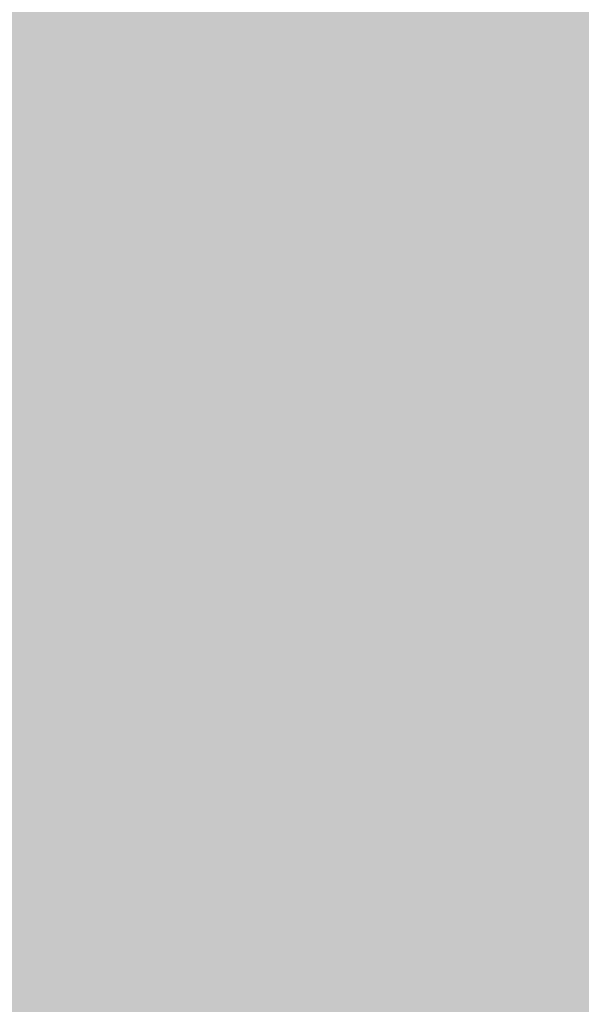
# Model space of a CAD drawing. Units: inches. Extents: x 2083 to 3317, y 1141 to 2115.
# Tile 177 of 256: x 3126.89136 to 3126.92826, y 1263.29018 to 1263.35483. Entities that reach past the tile are written whole.
import ezdxf

# ---------------------------------------------------------------- set-up
doc = ezdxf.new("R2010")
doc.units = ezdxf.units.IN
doc.layers.add('A-ANNO-DIMS', color=2, linetype='Continuous', lineweight=18)
doc.layers.add('A-WALL-PATT', color=251, linetype='Continuous', lineweight=13, true_color=0x636466)
doc.styles.get("Standard").update_dxf_attribs({"font": 'arial.ttf'})
doc.dimstyles.new('ISO-25', dxfattribs={"dimtxt": 12, "dimasz": 12, "dimexe": 1.25, "dimexo": 0.625, "dimtad": 1, "dimlunit": 3, "dimtxsty": 'Standard', "dimcen": 2.5, "dimadec": 0, "dimazin": 0, "dimtfac": 1, "dimtmove": 0, "dimatfit": 3, "dimfxl": 1, "dimarcsym": 0})

# ---------------------------------------------------------------- blocks, each defined once
blk = doc.blocks.new('*D26')
at = {"layer": 'A-ANNO-DIMS', "color": 0, "lineweight": -2, "transparency": 16777216}
for p, q in [((3088.985844, 1274.915092), (3088.985844, 1270.951963)), ((3111.240037, 1274.915092), (3111.240037, 1270.951963)), ((3076.985844, 1272.201963), (2840.262447, 1272.201963)), ((3111.240037, 1272.201963), (3088.985844, 1272.201963)), ((3123.240037, 1272.201963), (3135.240037, 1272.201963))]:
    blk.add_line(p, q, dxfattribs=at)
at = {"layer": 'A-ANNO-DIMS', "color": 0, "transparency": 16777216}
for points in [[(3076.985844, 1274.201963), (3076.985844, 1270.201963), (3088.985844, 1272.201963)], [(3123.240037, 1274.201963), (3123.240037, 1270.201963), (3111.240037, 1272.201963)]]:
    blk.add_solid(points, dxfattribs=at)
at = {"layer": 'Defpoints', "color": 0, "transparency": 16777216}
for p in [(3088.985844, 1275.540092), (3111.240037, 1275.540092), (3088.985844, 1272.201963)]:
    blk.add_point(p, dxfattribs=at)
at = {"layer": 'A-ANNO-DIMS', "color": 0, "transparency": 16777216, "insert": (2952.624146, 1279.031602), "char_height": 12, "attachment_point": 5}
blk.add_mtext('NIGHTSTAND 1\'-10 1/2" TYP.', dxfattribs=at)
blk = doc.blocks.new('*D27')
at = {"layer": 'A-ANNO-DIMS', "color": 0, "lineweight": -2, "transparency": 16777216}
for p, q in [((3114.578165, 1309.794285), (3114.578165, 1321.794285)), ((3111.865037, 1297.794285), (3115.828165, 1297.794285)), ((3114.578165, 1297.794285), (3114.578165, 1275.540092)), ((3111.865037, 1275.540092), (3115.828165, 1275.540092)), ((3114.578165, 1263.540092), (3114.578165, 1140.988591))]:
    blk.add_line(p, q, dxfattribs=at)
at = {"layer": 'A-ANNO-DIMS', "color": 0, "transparency": 16777216}
for points in [[(3112.578165, 1309.794285), (3116.578165, 1309.794285), (3114.578165, 1297.794285)], [(3112.578165, 1263.540092), (3116.578165, 1263.540092), (3114.578165, 1275.540092)]]:
    blk.add_solid(points, dxfattribs=at)
at = {"layer": 'Defpoints', "color": 0, "transparency": 16777216}
for p in [(3111.240037, 1297.794285), (3111.240037, 1275.540092), (3114.578165, 1275.540092)]:
    blk.add_point(p, dxfattribs=at)
at = {"layer": 'A-ANNO-DIMS', "color": 0, "transparency": 16777216, "insert": (3107.748527, 1196.264342), "char_height": 12, "attachment_point": 5, "rotation": 90}
blk.add_mtext('1\'-10 1/2" TYP.', dxfattribs=at)

msp = doc.modelspace()

# ---------------------------------------------------------------- hatches: boundary and pattern name
at = {"layer": 'A-WALL-PATT'}
h = msp.add_hatch(color=256, dxfattribs=at)
h.dxf.hatch_style = 1
h.paths.add_polyline_path([(3126.959783, 2020.76136), (2748.959783, 2020.76136), (2604.959783, 2020.76136), (2226.959783, 2020.76136), (2226.959783, 1702.76136), (2466.959783, 1702.76136), (2466.959783, 1582.76136), (2418.959783, 1582.76136), (2418.959783, 1477.76136), (2226.959783, 1477.76136), (2226.959783, 1263.26136), (2544.959783, 1263.26136), (2544.959783, 1411.76136), (2604.959783, 1411.76136), (2685.959783, 1411.76136), (2685.959783, 1420.76136), (2604.959783, 1420.76136), (2604.959783, 1573.76136), (2604.959783, 1702.76136), (2604.959783, 2011.76136), (2748.959783, 2011.76136), (2748.959783, 1702.76136), (2862.959783, 1702.76136), (2862.959783, 1621.76136), (2871.959783, 1621.76136), (2871.959783, 1702.76136), (2883.959783, 1702.76136), (2883.959783, 1706.939459, -0.026459), (2883.959783, 1711.76136), (2757.959783, 1711.76136), (2757.959783, 1807.76136), (2787.959783, 1807.76136), (2787.959783, 1812.26136), (2757.959783, 1812.26136), (2757.959783, 2011.76136), (2877.959783, 2011.76136), (2877.959783, 1812.26136), (2847.959783, 1812.26136), (2847.959783, 1807.76136), (2889.835742, 1807.76136), (2889.835742, 1812.26136), (2882.459783, 1812.26136), (2882.459783, 2011.76136), (3117.959783, 2011.76136), (3117.959783, 1812.26136), (2937.835742, 1812.26136), (2937.835742, 1807.76136), (2995.709783, 1807.76136), (2995.709783, 1796.117666), (3000.209783, 1796.117666), (3000.209783, 1807.76136), (3117.959783, 1807.76136), (3117.959783, 1711.76136), (3000.209783, 1711.76136), (3000.209783, 1760.117666), (2998.572705, 1760.117666, -0.020711), (2995.709783, 1760.117666), (2995.709783, 1711.76136), (2931.959783, 1711.76136), (2931.959783, 1702.76136), (3126.959783, 1702.76136)])
h.paths.add_polyline_path([(2471.459783, 2011.76136), (2471.459783, 1810.01136), (2462.716936, 1810.01136), (2462.716936, 1805.51136), (2505.959783, 1805.51136), (2505.959783, 1810.01136), (2475.959783, 1810.01136), (2475.959783, 2011.76136), (2595.959783, 2011.76136), (2595.959783, 1810.01136), (2565.959783, 1810.01136), (2565.959783, 1805.51136), (2595.959783, 1805.51136), (2595.959783, 1711.76136), (2235.959783, 1711.76136), (2235.959783, 1805.51136), (2353.709783, 1805.51136), (2353.709783, 1796.054162), (2358.209783, 1796.054162), (2358.209783, 1805.51136), (2414.716936, 1805.51136), (2414.716936, 1810.01136), (2235.959783, 1810.01136), (2235.959783, 2011.76136)], flags=16)
h.paths.add_polyline_path([(2270.204734, 1994.610008), (2270.204734, 1970.610008), (2246.204734, 1970.610008), (2246.204734, 1994.610008)], flags=0)
edge = h.paths.add_edge_path(flags=0)
edge.add_ellipse((2332.027391, 1899.798176), major_axis=(-3.042994, 3.042994), ratio=0.16825245, start_angle=-161.332166, end_angle=-156.307114, ccw=False)
edge.add_ellipse((2333.082037, 1898.74353), major_axis=(-1.054646, 1.054646), ratio=0.4535321, start_angle=-123.371019, end_angle=-94.159107)
edge = h.paths.add_edge_path(flags=0)
edge.add_ellipse((2332.027391, 1968.87629), major_axis=(3.042994, 3.042994), ratio=0.16825245, start_angle=18.667834, end_angle=23.692886)
edge.add_spline(control_points=[(2332.925596, 1970.691105), (2332.226768, 1970.3361), (2330.893709, 1969.658905), (2328.41308, 1970.932138), (2327.203934, 1967.748712), (2324.709596, 1969.955589), (2322.532822, 1967.012354), (2320.012846, 1971.295812), (2317.680308, 1968.157845), (2316.040526, 1967.102047), (2315.426904, 1966.809602)], knot_values=[0, 0, 0, 0, 2.267059, 4.324559, 6.685584, 8.878641, 11.121502, 14.300359, 17.755284, 19.732645, 19.732645, 19.732645, 19.732645], degree=3, periodic=0)
edge.add_ellipse((2332.027391, 1968.87629), major_axis=(3.042994, 3.042994), ratio=0.16825245, start_angle=18.667834, end_angle=23.692886, ccw=False)
edge.add_ellipse((2333.082037, 1969.930936), major_axis=(1.054646, 1.054646), ratio=0.4535321, start_angle=56.628981, end_angle=85.840893, ccw=False)
edge = h.paths.add_edge_path(flags=0)
edge.add_spline(control_points=[(2296.428287, 1967.987908), (2293.627804, 1965.336314), (2287.703624, 1959.727094), (2299.74386, 1949.995699), (2294.532591, 1935.668528), (2290.573228, 1920.603512), (2293.394124, 1909.973691), (2296.185407, 1904.966543)], knot_values=[0.099185, 0.099185, 0.099185, 0.099185, 0.345301, 0.619822, 0.982653, 1.386093, 1.810555, 1.810555, 1.810555, 1.810555], degree=3, periodic=0)
edge.add_spline(control_points=[(2296.185407, 1904.966543), (2297.383582, 1902.6193), (2298.000969, 1901.949312), (2298.55297, 1901.468155)], knot_values=[0.006246, 0.006246, 0.006246, 0.006246, 0.055476, 0.055476, 0.055476, 0.055476], degree=3, periodic=0)
edge.add_spline(control_points=[(2298.55297, 1901.468155), (2297.258612, 1900.923224), (2295.225294, 1900.232126), (2293.060229, 1900.614205), (2292.101423, 1900.788415), (2292.089578, 1900.790568)], knot_values=[0.312835, 0.312835, 0.312835, 0.312835, 0.40178, 0.474987, 0.475903, 0.475903, 0.475903, 0.475903], degree=3, periodic=0)
edge.add_arc((2292.793646, 1904.664109), 3.937008, 215.420897, 259.698179, ccw=False)
edge.add_spline(control_points=[(2289.585314, 1902.382304), (2289.476652, 1902.535087), (2289.36848, 1902.688035), (2289.260865, 1902.84117)], knot_values=[0.102872, 0.102872, 0.102872, 0.102872, 0.116896, 0.116896, 0.116896, 0.116896], degree=3, periodic=0)
edge.add_spline(control_points=[(2289.260865, 1902.84117), (2288.686604, 1902.550192), (2287.640048, 1902.019902), (2285.881337, 1901.873954), (2283.852972, 1901.504352), (2281.719987, 1899.710538), (2278.466991, 1899.492942), (2276.157136, 1901.883202), (2272.258953, 1899.804071), (2267.777605, 1901.843183), (2262.243882, 1900.184033), (2257.414927, 1901.782061), (2254.318374, 1900.72612), (2253.178285, 1900.337343)], knot_values=[0, 0, 0, 0, 1.907977, 3.477176, 5.261074, 7.972851, 11.680248, 13.717921, 16.939592, 22.789562, 27.502503, 33.595215, 37.145618, 37.145618, 37.145618, 37.145618], degree=3, periodic=0)
edge.add_line((2253.178285, 1900.337343), (2250.24424, 1902.84117))
edge.add_line((2250.24424, 1902.84117), (2250.24424, 1965.833296))
edge.add_line((2250.24424, 1965.833296), (2253.178285, 1968.337123))
edge.add_spline(control_points=[(2253.178285, 1968.337123), (2254.318374, 1967.948346), (2257.414927, 1966.892405), (2262.243882, 1968.490433), (2267.777605, 1966.831283), (2271.52673, 1968.537217), (2273.875914, 1967.828289), (2274.206701, 1967.727642)], knot_values=[0, 0, 0, 0, 0.09018, 0.244935, 0.364644, 0.513233, 0.537855, 0.537855, 0.537855, 0.537855], degree=3, periodic=0)
edge.add_arc((2274.352887, 1963.793349), 3.937008, 72.051134, 92.127949, ccw=False)
edge.add_arc((2281.296933, 1985.230003), 18.596298, 252.0511336, 288.5657217)
edge.add_arc((2292.316717, 1956.02888), 12.646081, 71.0267879, 113.7782184, ccw=False)
edge = h.paths.add_edge_path(flags=0)
edge.add_spline(control_points=[(2274.899415, 1951.856195), (2275.066156, 1951.616592), (2275.232687, 1951.376588), (2275.397987, 1951.135855)], knot_values=[1.409916, 1.409916, 1.409916, 1.409916, 1.43159, 1.43159, 1.43159, 1.43159], degree=3, periodic=0)
edge.add_spline(control_points=[(2275.397987, 1951.135855), (2275.792106, 1950.561885), (2276.179231, 1949.983774), (2276.545546, 1949.397103)], knot_values=[1.358238, 1.358238, 1.358238, 1.358238, 1.409916, 1.409916, 1.409916, 1.409916], degree=3, periodic=0)
edge.add_line((2276.545546, 1949.397103), (2277.437289, 1947.862185))
edge.add_spline(control_points=[(2277.437289, 1947.862185), (2276.303834, 1945.673115), (2274.639698, 1942.426882), (2274.631615, 1938.0939), (2272.799124, 1930.85155), (2274.356426, 1943.897046), (2275.947681, 1947.923356), (2276.545546, 1949.397103)], knot_values=[0.005632, 0.005632, 0.005632, 0.005632, 0.186014, 0.266002, 0.357087, 0.59639, 0.739732, 0.739732, 0.739732, 0.739732], degree=3, periodic=0)
edge.add_spline(control_points=[(2276.545546, 1949.397103), (2276.179231, 1949.983774), (2275.792106, 1950.561885), (2275.397987, 1951.135855)], knot_values=[1.358238, 1.358238, 1.358238, 1.358238, 1.409916, 1.409916, 1.409916, 1.409916], degree=3, periodic=0)
edge.add_spline(control_points=[(2275.397987, 1951.135855), (2274.9425, 1950.080452), (2274.20776, 1948.025272), (2273.934602, 1944.851477), (2272.468534, 1937.627489), (2273.466216, 1945.696466), (2274.700615, 1951.059472), (2274.899415, 1951.856195)], knot_values=[0.104364, 0.104364, 0.104364, 0.104364, 0.189636, 0.269624, 0.36071, 0.600013, 0.644622, 0.644622, 0.644622, 0.644622], degree=3, periodic=0)
h.paths.add_polyline_path([(2269.167514, 1963.127573, -0.357527), (2268.170633, 1960.97637, -0.092561), (2268.170633, 1939.436325, -0.357527), (2269.167514, 1937.285122, -0.357527), (2267.01631, 1938.282002, -0.164785), (2254.685581, 1938.282002, -0.357527), (2252.534378, 1937.285122, -0.357527), (2253.531259, 1939.436325, -0.092561), (2253.531259, 1960.97637, -0.357527), (2252.534378, 1963.127573, -0.357527), (2254.685581, 1962.130692, -0.164785), (2267.01631, 1962.130692, -0.357527)], flags=0)
h.paths.add_polyline_path([(2248.874068, 1967.8018), (2248.874068, 1957.02771), (2249.457783, 1957.02771), (2249.457783, 1911.646756), (2248.874068, 1911.646756), (2248.874068, 1900.872666), (2246.511863, 1900.872666, 0.197327), (2244.149658, 1902.456873), (2244.149658, 1966.217592, 0.197327), (2246.511863, 1967.8018)], flags=0)
h.paths.add_polyline_path([(2269.167514, 1931.389344, -0.357527), (2268.170633, 1929.238141, -0.092561), (2268.170633, 1907.698096, -0.357527), (2269.167514, 1905.546893, -0.357527), (2267.01631, 1906.543774, -0.164785), (2254.685581, 1906.543774, -0.357527), (2252.534378, 1905.546893, -0.357527), (2253.531259, 1907.698096, -0.092561), (2253.531259, 1929.238141, -0.357527), (2252.534378, 1931.389344, -0.357527), (2254.685581, 1930.392463, -0.164785), (2267.01631, 1930.392463, -0.357527)], flags=0)
edge = h.paths.add_edge_path(flags=0)
edge.add_spline(control_points=[(2276.196858, 1906.723702), (2276.168144, 1909.028928), (2276.114049, 1913.371852), (2270.598417, 1924.924978), (2273.905175, 1919.012779), (2275.921711, 1916.262063), (2275.47457, 1912.402149), (2277.257874, 1910.380621), (2276.696044, 1908.225036), (2276.646218, 1906.813023), (2276.617825, 1906.008407)], knot_values=[0, 0, 0, 0, 8.61026, 16.221274, 18.843057, 23.804898, 27.440828, 29.356102, 31.203478, 33.650687, 33.650687, 33.650687, 33.650687], degree=3, periodic=0)
edge.add_spline(control_points=[(2276.617825, 1906.008407), (2276.623313, 1905.624144), (2276.497738, 1904.628661), (2275.441779, 1903.854725), (2274.937314, 1903.08045), (2274.85908, 1902.84117)], knot_values=[0.156488, 0.156488, 0.156488, 0.156488, 0.184398, 0.231376, 0.250598, 0.250598, 0.250598, 0.250598], degree=3, periodic=0)
edge.add_line((2274.85908, 1902.84117), (2276.50598, 1902.84117))
edge.add_spline(control_points=[(2276.50598, 1902.84117), (2276.788308, 1903.08494), (2277.665071, 1904.125196), (2278.249538, 1904.340738), (2277.653872, 1908.527387), (2278.15567, 1906.227808), (2278.100464, 1905.285948), (2278.846675, 1904.069005), (2277.856785, 1903.414948), (2277.874191, 1902.99105), (2277.903562, 1902.84117)], knot_values=[0.059574, 0.059574, 0.059574, 0.059574, 0.080753, 0.103741, 0.16972, 0.176036, 0.207137, 0.240474, 0.262341, 0.27366, 0.27366, 0.27366, 0.27366], degree=3, periodic=0)
edge.add_line((2277.903562, 1902.84117), (2280.029825, 1902.84117))
edge.add_spline(control_points=[(2280.029825, 1902.84117), (2279.888221, 1903.088398), (2279.499257, 1903.981551), (2280.152284, 1905.939349), (2278.103615, 1909.657757), (2279.762395, 1907.185285), (2280.3279, 1904.874861), (2280.485109, 1903.48959), (2281.463269, 1903.249432), (2281.758343, 1902.936497), (2281.834036, 1902.84117)], knot_values=[0.013856, 0.013856, 0.013856, 0.013856, 0.034874, 0.088867, 0.107879, 0.126738, 0.158714, 0.193757, 0.217487, 0.226722, 0.226722, 0.226722, 0.226722], degree=3, periodic=0)
edge.add_spline(control_points=[(2281.834036, 1902.84117), (2281.787535, 1902.826703), (2281.647022, 1902.782988), (2281.395527, 1902.85949), (2281.088077, 1902.985242), (2280.720683, 1903.060902), (2280.333451, 1903.025726), (2280.124767, 1902.898879), (2280.029825, 1902.84117)], knot_values=[0, 0, 0, 0, 0.14413, 0.435517, 0.749276, 1.153046, 1.548371, 1.878348, 1.878348, 1.878348, 1.878348], degree=3, periodic=0)
edge.add_line((2280.029825, 1902.84117), (2277.903562, 1902.84117))
edge.add_spline(control_points=[(2277.903562, 1902.84117), (2277.892855, 1902.795855), (2277.865396, 1902.679637), (2277.607479, 1902.687483), (2277.27405, 1902.8007), (2276.837921, 1902.619775), (2276.583807, 1902.789261), (2276.50598, 1902.84117)], knot_values=[0, 0, 0, 0, 0.127189, 0.326199, 0.628009, 1.24357, 1.515331, 1.515331, 1.515331, 1.515331], degree=3, periodic=0)
edge.add_line((2276.50598, 1902.84117), (2274.85908, 1902.84117))
edge.add_spline(control_points=[(2274.85908, 1902.84117), (2274.814437, 1902.898587), (2274.72513, 1903.013446), (2274.493477, 1903.118968), (2274.244285, 1902.960539), (2273.937121, 1903.184942), (2273.614039, 1902.983143), (2273.408316, 1902.883045), (2273.322254, 1902.84117)], knot_values=[0, 0, 0, 0, 0.21843, 0.436957, 0.687977, 0.990379, 1.398396, 1.69185, 1.69185, 1.69185, 1.69185], degree=3, periodic=0)
edge.add_spline(control_points=[(2273.322254, 1902.84117), (2273.61674, 1903.445692), (2274.273998, 1904.538253), (2276.027239, 1904.573702), (2276.206963, 1906.583637), (2276.196858, 1906.723702)], knot_values=[0.012227, 0.012227, 0.012227, 0.012227, 0.059472, 0.106218, 0.134458, 0.134458, 0.134458, 0.134458], degree=3, periodic=0)
h.paths.add_polyline_path([(2270.776054, 1897.789828), (2270.776054, 1873.789828), (2246.776054, 1873.789828), (2246.776054, 1897.789828)], flags=0)
h.paths.add_polyline_path([(2353.709783, 1760.005059), (2353.709783, 1760.054162), (2358.209783, 1760.054162, -0.033729)], flags=0)
h.paths.add_polyline_path([(2321.819119, 1737.529186), (2341.995327, 1737.529186, -0.414214), (2343.203273, 1736.321241), (2343.203273, 1721.020596, -0.414214), (2341.995327, 1719.812651), (2321.819119, 1719.812651, -0.414214), (2320.611173, 1721.020596), (2320.611173, 1736.321241, -0.414214)], flags=0)
h.paths.add_polyline_path([(2324.23501, 1736.321241), (2339.579436, 1736.321241, -0.414214), (2341.995327, 1733.905349), (2341.995327, 1725.44973, -0.414214), (2339.579436, 1723.033839), (2333.680588, 1723.033839), (2333.845317, 1722.045467, -0.870646), (2335.425399, 1721.825893, -0.767327), (2333.922694, 1721.423245), (2331.291024, 1721.423245, -0.767327), (2329.788319, 1721.825893, -0.870646), (2331.368401, 1722.045467), (2331.53313, 1723.033839), (2324.23501, 1723.033839, -0.414214), (2321.819119, 1725.44973), (2321.819119, 1733.905349, -0.414214)], flags=0)
h.paths.add_polyline_path([(2570.483789, 1928.615444), (2589.683789, 1928.615444), (2590.168829, 1928.615444), (2590.168829, 1904.993397), (2570.483789, 1904.993397)], flags=0)
h.paths.add_polyline_path([(2574.447324, 1927.263822, -1), (2572.828836, 1927.263822, -1)], flags=0)
h.paths.add_polyline_path([(2573.089867, 1926.940877), (2573.925032, 1927.776042), (2574.147743, 1927.553332), (2573.312577, 1926.718166)], flags=0)
h.paths.add_polyline_path([(2578.779065, 1919.729618, -1), (2571.591663, 1919.729618, -1)], flags=0)
h.paths.add_polyline_path([(2578.385364, 1919.729618, -1), (2571.985364, 1919.729618, -1)], flags=0)
h.paths.add_polyline_path([(2331.595764, 1729.476216, -1), (2333.617954, 1729.476216, -1)], flags=0)
h.paths.add_polyline_path([(2578.034228, 1927.263822, -1), (2576.41574, 1927.263822, -1)], flags=0)
h.paths.add_polyline_path([(2576.688851, 1927.531089), (2576.911562, 1927.753799), (2577.746728, 1926.918634), (2577.524017, 1926.695923)], flags=0)
h.paths.add_polyline_path([(2578.139065, 1909.859539, -1), (2572.231663, 1909.859539, -1)], flags=0)
h.paths.add_polyline_path([(2577.745364, 1909.859539, -1), (2572.625364, 1909.859539, -1)], flags=0)
h.paths.add_polyline_path([(2583.797718, 1927.263822, -1), (2582.179229, 1927.263822, -1)], flags=0)
h.paths.add_polyline_path([(2582.718649, 1927.753799), (2583.553814, 1926.918634), (2583.331103, 1926.695923), (2582.495938, 1927.531089)], flags=0)
h.paths.add_polyline_path([(2582.495938, 1927.531089), (2582.718649, 1927.753799), (2583.553814, 1926.918634), (2583.331103, 1926.695923)], flags=0)
h.paths.add_polyline_path([(2587.739065, 1920.529618, -1), (2581.831663, 1920.529618, -1)], flags=0)
h.paths.add_polyline_path([(2587.345364, 1920.529618, -1), (2582.225364, 1920.529618, -1)], flags=0)
h.paths.add_polyline_path([(2587.384622, 1927.263822, -1), (2585.766133, 1927.263822, -1)], flags=0)
h.paths.add_polyline_path([(2586.081993, 1926.980247), (2586.917158, 1927.815412), (2587.139869, 1927.592702), (2586.304703, 1926.757536)], flags=0)
h.paths.add_polyline_path([(2588.379065, 1910.659539, -1), (2581.191663, 1910.659539, -1)], flags=0)
h.paths.add_polyline_path([(2587.985364, 1910.659539, -1), (2581.585364, 1910.659539, -1)], flags=0)
h.paths.add_polyline_path([(2417.167729, 1729.477895), (2437.343937, 1729.477895, -0.414214), (2438.551883, 1728.26995), (2438.551883, 1712.969306, -0.414214), (2437.343937, 1711.76136), (2417.167729, 1711.76136, -0.414214), (2415.959783, 1712.969306), (2415.959783, 1728.26995, -0.414214)], flags=0)
h.paths.add_polyline_path([(2419.58362, 1728.26995), (2434.928046, 1728.26995, -0.414214), (2437.343937, 1725.854059), (2437.343937, 1717.39844, -0.414214), (2434.928046, 1714.982548), (2429.029199, 1714.982548), (2429.193927, 1713.994176, -0.870646), (2430.774009, 1713.774603, -0.767327), (2429.271304, 1713.371954), (2426.639634, 1713.371954, -0.767327), (2425.136929, 1713.774603, -0.870646), (2426.717011, 1713.994176), (2426.88174, 1714.982548), (2419.58362, 1714.982548, -0.414214), (2417.167729, 1717.39844), (2417.167729, 1725.854059, -0.414214)], flags=0)
h.paths.add_polyline_path([(2419.58362, 1728.26995), (2434.928046, 1728.26995, -0.414214), (2437.343937, 1725.854059), (2437.343937, 1717.39844, -0.414214), (2434.928046, 1714.982548), (2429.029199, 1714.982548), (2428.358118, 1719.009034), (2427.552821, 1719.009034), (2426.88174, 1714.982548), (2419.58362, 1714.982548, -0.414214), (2417.167729, 1717.39844), (2417.167729, 1725.854059, -0.414214)], flags=0)
h.paths.add_polyline_path([(2426.944374, 1721.424925, -1), (2428.966564, 1721.424925, -1)], flags=0)
h.paths.add_polyline_path([(2475.959783, 1702.76136), (2595.959783, 1702.76136), (2595.959783, 1582.76136), (2475.959783, 1582.76136)], flags=16)
h.paths.add_polyline_path([(2427.959783, 1573.76136), (2595.959783, 1573.76136), (2595.959783, 1468.76136), (2595.959783, 1420.76136), (2384.459783, 1420.76136), (2384.459783, 1468.76136), (2427.959783, 1468.76136)], flags=16)
h.paths.add_polyline_path([(2379.959783, 1468.76136), (2379.959783, 1420.76136), (2235.959783, 1420.76136), (2235.959783, 1468.76136)], flags=16)
h.paths.add_polyline_path([(2317.815996, 1466.695767), (2337.992205, 1466.695767, -0.414214), (2339.20015, 1465.487821), (2339.20015, 1450.187177, -0.414214), (2337.992205, 1448.979232), (2317.815996, 1448.979232, -0.414214), (2316.608051, 1450.187177), (2316.608051, 1465.487821, -0.414214)], flags=0)
h.paths.add_polyline_path([(2320.231887, 1465.487821), (2335.576313, 1465.487821, -0.414214), (2337.992205, 1463.07193), (2337.992205, 1454.616311, -0.414214), (2335.576313, 1452.20042), (2329.677466, 1452.20042), (2329.842195, 1451.212047, -0.870646), (2331.422276, 1450.992474, -0.767327), (2329.919571, 1450.589826), (2327.287902, 1450.589826, -0.767327), (2325.785197, 1450.992474, -0.870646), (2327.365278, 1451.212047), (2327.530007, 1452.20042), (2320.231887, 1452.20042, -0.414214), (2317.815996, 1454.616311), (2317.815996, 1463.07193, -0.414214)], flags=0)
h.paths.add_polyline_path([(2320.231887, 1465.487821), (2335.576313, 1465.487821, -0.414214), (2337.992205, 1463.07193), (2337.992205, 1454.616311, -0.414214), (2335.576313, 1452.20042), (2329.677466, 1452.20042), (2329.006385, 1456.226905), (2328.201088, 1456.226905), (2327.530007, 1452.20042), (2320.231887, 1452.20042, -0.414214), (2317.815996, 1454.616311), (2317.815996, 1463.07193, -0.414214)], flags=0)
h.paths.add_polyline_path([(2327.592641, 1458.642796, -1), (2329.614832, 1458.642796, -1)], flags=0)
h.paths.add_polyline_path([(2244.411744, 1433.340453), (2241.920945, 1433.340453, -0.414214), (2240.017856, 1435.243542), (2240.017856, 1440.952808, -0.414211), (2241.920925, 1442.855897), (2244.411744, 1442.855897, -1.976472)], flags=0)
h.paths.add_polyline_path([(2245.356888, 1434.397536, -0.414214), (2245.356888, 1441.798814, -2.144098)], flags=0)
h.paths.add_polyline_path([(2535.959783, 1416.26136), (2535.959783, 1272.26136), (2235.959783, 1272.26136), (2235.959783, 1416.26136)], flags=16)
h.paths.add_polyline_path([(2260.119561, 1384.292841), (2260.119561, 1362.038649), (2237.865369, 1362.038649), (2237.865369, 1384.292841)], flags=0)
edge = h.paths.add_edge_path(flags=0)
edge.add_line((2318.251847, 1362.093298), (2318.145797, 1362.000973))
edge.add_ellipse((2317.445116, 1360.431044), major_axis=(2.82164, 2.82164), ratio=0.16825245, start_angle=18.667834, end_angle=20.948127, ccw=False)
edge.add_ellipse((2318.423045, 1361.408974), major_axis=(0.977929, 0.977929), ratio=0.4535321, start_angle=56.628981, end_angle=70.226201, ccw=False)
edge = h.paths.add_edge_path(flags=0)
edge.add_line((2319.10737, 1295.571078), (2319.015044, 1295.677128))
edge.add_ellipse((2317.445116, 1296.377809), major_axis=(-2.82164, 2.82164), ratio=0.16825245, start_angle=-161.332166, end_angle=-159.051873, ccw=False)
edge.add_ellipse((2318.423045, 1295.39988), major_axis=(-0.977929, 0.977929), ratio=0.4535321, start_angle=-123.371019, end_angle=-109.773799)
edge = h.paths.add_edge_path(flags=0)
edge.add_spline(control_points=[(2284.210349, 1301.170219), (2284.580688, 1300.444719), (2284.891189, 1299.892024), (2285.159553, 1299.461018)], knot_values=[0.039066, 0.039066, 0.039066, 0.039066, 0.055476, 0.055476, 0.055476, 0.055476], degree=3, periodic=0)
edge.add_line((2285.159553, 1299.461018), (2284.210349, 1301.170219))
edge = h.paths.add_edge_path(flags=0)
edge.add_line((2280.412458, 1297.298013), (2283.369991, 1297.036122))
edge.add_line((2283.369991, 1297.036122), (2286.40569, 1297.92631))
edge.add_spline(control_points=[(2286.40569, 1297.92631), (2285.305487, 1297.463119), (2284.344777, 1297.129151), (2283.369991, 1297.036122)], knot_values=[0.394369, 0.394369, 0.394369, 0.394369, 0.475903, 0.475903, 0.475903, 0.475903], degree=3, periodic=0)
edge.add_spline(control_points=[(2283.369991, 1297.036122), (2283.28139, 1297.027666), (2282.316289, 1296.957336), (2281.312502, 1297.134479), (2280.423441, 1297.296016), (2280.412458, 1297.298013)], knot_values=[0.312835, 0.312835, 0.312835, 0.312835, 0.320246, 0.393453, 0.394369, 0.394369, 0.394369, 0.394369], degree=3, periodic=0)
edge = h.paths.add_edge_path(flags=0)
edge.add_line((2284.435561, 1359.607285), (2280.446291, 1355.328047))
edge.add_line((2280.446291, 1355.328047), (2279.579987, 1351.017754))
edge.add_line((2279.579987, 1351.017754), (2282.412974, 1346.580433))
edge.add_spline(control_points=[(2282.412974, 1346.580433), (2283.153331, 1345.589236), (2284.252896, 1344.028897), (2284.801037, 1342.387167), (2284.935162, 1341.805544)], knot_values=[1.240098, 1.240098, 1.240098, 1.240098, 1.332892, 1.382712, 1.382712, 1.382712, 1.382712], degree=3, periodic=0)
edge.add_spline(control_points=[(2284.935162, 1341.805544), (2285.319108, 1340.1406), (2285.233029, 1338.409204), (2284.909938, 1336.654122)], knot_values=[1.097484, 1.097484, 1.097484, 1.097484, 1.240098, 1.240098, 1.240098, 1.240098], degree=3, periodic=0)
edge.add_spline(control_points=[(2284.909938, 1336.654122), (2284.586848, 1334.89904), (2284.026745, 1333.120272), (2283.462644, 1331.360585)], knot_values=[0.95487, 0.95487, 0.95487, 0.95487, 1.097484, 1.097484, 1.097484, 1.097484], degree=3, periodic=0)
edge.add_line((2283.462644, 1331.360585), (2281.890376, 1326.153357))
edge.add_line((2281.890376, 1326.153357), (2280.756259, 1321.056089))
edge.add_line((2280.756259, 1321.056089), (2280.299205, 1316.001977))
edge.add_line((2280.299205, 1316.001977), (2280.715933, 1310.950068))
edge.add_line((2280.715933, 1310.950068), (2282.028094, 1305.972137))
edge.add_line((2282.028094, 1305.972137), (2284.210349, 1301.170219))
edge.add_spline(control_points=[(2284.210349, 1301.170219), (2283.340731, 1302.730185), (2282.611904, 1304.336493), (2282.028094, 1305.972137)], knot_values=[0.099185, 0.099185, 0.099185, 0.099185, 0.241799, 0.241799, 0.241799, 0.241799], degree=3, periodic=0)
edge.add_spline(control_points=[(2282.028094, 1305.972137), (2281.444283, 1307.60778), (2281.005489, 1309.272759), (2280.715933, 1310.950068)], knot_values=[0.241799, 0.241799, 0.241799, 0.241799, 0.384413, 0.384413, 0.384413, 0.384413], degree=3, periodic=0)
edge.add_spline(control_points=[(2280.715933, 1310.950068), (2280.433241, 1312.587613), (2280.289386, 1314.276959), (2280.298894, 1315.962032), (2280.299205, 1316.001977)], knot_values=[0.384413, 0.384413, 0.384413, 0.384413, 0.523647, 0.527028, 0.527028, 0.527028, 0.527028], degree=3, periodic=0)
edge.add_spline(control_points=[(2280.299205, 1316.001977), (2280.312326, 1317.686955), (2280.477871, 1319.367926), (2280.756259, 1321.056089)], knot_values=[0.527028, 0.527028, 0.527028, 0.527028, 0.669642, 0.669642, 0.669642, 0.669642], degree=3, periodic=0)
edge.add_spline(control_points=[(2280.756259, 1321.056089), (2281.034648, 1322.744252), (2281.42588, 1324.439608), (2281.890376, 1326.153357)], knot_values=[0.669642, 0.669642, 0.669642, 0.669642, 0.812256, 0.812256, 0.812256, 0.812256], degree=3, periodic=0)
edge.add_spline(control_points=[(2281.890376, 1326.153357), (2282.264383, 1327.533251), (2282.78787, 1329.26181), (2283.352751, 1331.01778), (2283.462644, 1331.360585)], knot_values=[0.812256, 0.812256, 0.812256, 0.812256, 0.927087, 0.95487, 0.95487, 0.95487, 0.95487], degree=3, periodic=0)
edge.add_line((2283.462644, 1331.360585), (2284.909938, 1336.654122))
edge.add_line((2284.909938, 1336.654122), (2284.935162, 1341.805544))
edge.add_line((2284.935162, 1341.805544), (2282.412974, 1346.580433))
edge.add_spline(control_points=[(2282.412974, 1346.580433), (2281.275127, 1348.103792), (2280.078447, 1349.570318), (2279.579987, 1351.017754)], knot_values=[1.382712, 1.382712, 1.382712, 1.382712, 1.525326, 1.525326, 1.525326, 1.525326], degree=3, periodic=0)
edge.add_spline(control_points=[(2279.579987, 1351.017754), (2279.443282, 1351.414721), (2279.136312, 1352.856922), (2279.73519, 1354.290385), (2280.446291, 1355.328047)], knot_values=[1.525326, 1.525326, 1.525326, 1.525326, 1.564439, 1.667941, 1.667941, 1.667941, 1.667941], degree=3, periodic=0)
edge.add_spline(control_points=[(2280.446291, 1355.328047), (2281.426113, 1356.757835), (2282.930837, 1358.18256), (2284.435561, 1359.607285)], knot_values=[1.667941, 1.667941, 1.667941, 1.667941, 1.810555, 1.810555, 1.810555, 1.810555], degree=3, periodic=0)
edge.add_arc((2280.623075, 1348.518181), 11.72618, 71.0267879, 113.7782184)
edge.add_arc((2270.404892, 1375.595156), 17.243567, 252.0511336, 288.5657217, ccw=False)
edge.add_arc((2263.965969, 1355.717847), 3.650622, 72.051134, 92.127949)
edge.add_arc((2263.965969, 1355.717847), 3.650622, 92.127949, 177.98513)
edge.add_spline(control_points=[(2260.317604, 1355.846199), (2260.260417, 1354.220668), (2260.551278, 1350.186547), (2262.999344, 1346.766251), (2264.472741, 1344.649024)], knot_values=[1.43159, 1.43159, 1.43159, 1.43159, 1.564144, 1.770695, 1.770695, 1.770695, 1.770695], degree=3, periodic=0)
edge.add_line((2264.472741, 1344.649024), (2264.93559, 1343.98253))
edge.add_spline(control_points=[(2263.801044, 1340.248105), (2263.843238, 1340.514088), (2264.067244, 1341.756465), (2264.512693, 1343.002453), (2264.935047, 1343.981083)], knot_values=[0.53657, 0.53657, 0.53657, 0.53657, 0.559349, 0.644622, 0.644622, 0.644622, 0.644622], degree=3, periodic=0)
edge.add_spline(control_points=[(2264.935047, 1343.981083), (2265.117771, 1343.714975), (2265.298875, 1343.447906), (2265.476756, 1343.179365)], knot_values=[1.384077, 1.384077, 1.384077, 1.384077, 1.409916, 1.409916, 1.409916, 1.409916], degree=3, periodic=0)
edge.add_spline(control_points=[(2265.476756, 1343.179365), (2265.654637, 1342.910823), (2265.829296, 1342.64081), (2265.99913, 1342.368812)], knot_values=[1.358238, 1.358238, 1.358238, 1.358238, 1.384077, 1.384077, 1.384077, 1.384077], degree=3, periodic=0)
edge.add_line((2265.99913, 1342.368812), (2266.826006, 1340.945547))
edge.add_spline(control_points=[(2266.826006, 1340.945547), (2268.894401, 1337.089691), (2271.398173, 1325.843001), (2270.516164, 1310.568557), (2275.919376, 1301.860609), (2277.789511, 1299.19945)], knot_values=[0.116896, 0.116896, 0.116896, 0.116896, 0.472987, 1.050969, 1.313793, 1.313793, 1.313793, 1.313793], degree=3, periodic=0)
edge.add_spline(control_points=[(2277.789511, 1299.19945), (2277.839405, 1299.128452), (2277.889428, 1299.057498), (2277.939572, 1298.986584)], knot_values=[0.109884, 0.109884, 0.109884, 0.109884, 0.116896, 0.116896, 0.116896, 0.116896], degree=3, periodic=0)
edge.add_line((2277.939572, 1298.986584), (2277.788849, 1299.199114))
edge.add_spline(control_points=[(2277.788849, 1299.199114), (2277.256582, 1298.929414), (2276.28635, 1298.437902), (2275.039352, 1298.334419), (2274.38333, 1298.238895), (2274.215254, 1298.209338)], knot_values=[33.12187, 33.12187, 33.12187, 33.12187, 35.029056, 36.598255, 37.144827, 37.144827, 37.144827, 37.144827], degree=3, periodic=0)
edge.add_line((2274.215254, 1298.209338), (2273.073147, 1297.892961))
edge.add_spline(control_points=[(2273.073147, 1297.892961), (2272.322936, 1297.579784), (2271.039151, 1296.510508), (2269.248395, 1296.226062), (2268.4231, 1296.374654)], knot_values=[26.532584, 26.532584, 26.532584, 26.532584, 29.198919, 31.839101, 31.839101, 31.839101, 31.839101], degree=3, periodic=0)
edge.add_line((2268.4231, 1296.374654), (2263.878501, 1297.457534))
edge.add_spline(control_points=[(2263.878501, 1297.457534), (2263.556077, 1297.359435), (2261.860306, 1296.838694), (2260.23878, 1297.282407), (2258.933454, 1297.516461)], knot_values=[15.919551, 15.919551, 15.919551, 15.919551, 16.939592, 21.226067, 21.226067, 21.226067, 21.226067], degree=3, periodic=0)
edge.add_line((2258.933454, 1297.516461), (2254.055233, 1297.32901))
edge.add_spline(control_points=[(2254.055233, 1297.32901), (2253.755525, 1297.295815), (2252.113683, 1297.165174), (2250.461869, 1297.544221), (2249.129686, 1297.667882)], knot_values=[5.306517, 5.306517, 5.306517, 5.306517, 6.276435, 10.613034, 10.613034, 10.613034, 10.613034], degree=3, periodic=0)
edge.add_line((2249.129686, 1297.667882), (2244.33165, 1296.877756))
edge.add_line((2244.33165, 1296.877756), (2241.611033, 1299.19945))
edge.add_line((2241.611033, 1299.19945), (2241.611033, 1357.609404))
edge.add_line((2241.611033, 1357.609404), (2244.33165, 1359.931097))
edge.add_line((2244.33165, 1359.931097), (2252.728823, 1359.542692))
edge.add_spline(control_points=[(2252.728823, 1359.542692), (2252.870939, 1359.54644), (2253.30574, 1359.548172), (2253.739845, 1359.514274), (2254.031742, 1359.482426)], knot_values=[0.233291, 0.233291, 0.233291, 0.233291, 0.244935, 0.268927, 0.268927, 0.268927, 0.268927], degree=3, periodic=0)
edge.add_line((2254.031742, 1359.482426), (2259.58719, 1359.41639))
edge.add_spline(control_points=[(2259.58719, 1359.41639), (2260.677068, 1359.628503), (2262.073197, 1359.897003), (2263.523692, 1359.459278), (2263.830417, 1359.365952)], knot_values=[0.422516, 0.422516, 0.422516, 0.422516, 0.513233, 0.537855, 0.537855, 0.537855, 0.537855], degree=3, periodic=0)
edge.add_arc((2263.965969, 1355.717847), 3.650622, 72.051134, 92.127949, ccw=False)
edge.add_arc((2270.404892, 1375.595156), 17.243567, 252.0511336, 288.5657217)
edge.add_arc((2280.623075, 1348.518181), 11.72618, 71.0267879, 113.7782184, ccw=False)
h.paths.add_polyline_path([(2240.34053, 1359.434715), (2240.34053, 1349.444353), (2240.881785, 1349.444353), (2240.881785, 1307.3645), (2240.34053, 1307.3645), (2240.34053, 1297.374138), (2238.150157, 1297.374138, 0.197327), (2235.959783, 1298.843108), (2235.959783, 1357.965746, 0.197327), (2238.150157, 1359.434715)], flags=0)
h.paths.add_polyline_path([(2259.15779, 1355.1005, -0.357527), (2258.233425, 1353.10578, -0.092561), (2258.233425, 1333.132601, -0.357527), (2259.15779, 1331.13788, -0.357527), (2257.16307, 1332.062246, -0.164785), (2245.729302, 1332.062246, -0.357527), (2243.734582, 1331.13788, -0.357527), (2244.658947, 1333.132601, -0.092561), (2244.658947, 1353.10578, -0.357527), (2243.734582, 1355.1005, -0.357527), (2245.729302, 1354.176135, -0.164785), (2257.16307, 1354.176135, -0.357527)], flags=0)
edge = h.paths.add_edge_path(flags=0)
edge.add_line((2265.99913, 1342.368812), (2266.826006, 1340.945547))
edge.add_line((2266.826006, 1340.945547), (2265.307557, 1337.814066))
edge.add_line((2265.307557, 1337.814066), (2264.358232, 1334.652939))
edge.add_line((2264.358232, 1334.652939), (2264.262012, 1333.799705))
edge.add_spline(control_points=[(2264.262012, 1333.799705), (2264.208357, 1333.187055), (2264.16206, 1332.365525), (2264.007144, 1331.413933), (2263.969049, 1331.201834)], knot_values=[0.464444, 0.464444, 0.464444, 0.464444, 0.516691, 0.531608, 0.531608, 0.531608, 0.531608], degree=3, periodic=0)
edge.add_spline(control_points=[(2263.969049, 1331.201834), (2263.774535, 1330.118873), (2263.42437, 1328.790839), (2263.25742, 1328.530652), (2263.234028, 1328.514612)], knot_values=[0.372682, 0.372682, 0.372682, 0.372682, 0.44885, 0.464444, 0.464444, 0.464444, 0.464444], degree=3, periodic=0)
edge.add_spline(control_points=[(2263.234028, 1328.514612), (2263.096382, 1328.420227), (2263.13117, 1329.301477), (2263.274953, 1330.615749)], knot_values=[0.280919, 0.280919, 0.280919, 0.280919, 0.372682, 0.372682, 0.372682, 0.372682], degree=3, periodic=0)
edge.add_spline(control_points=[(2263.274953, 1330.615749), (2263.418736, 1331.930022), (2263.671515, 1333.677318), (2263.969852, 1335.315027)], knot_values=[0.189157, 0.189157, 0.189157, 0.189157, 0.280919, 0.280919, 0.280919, 0.280919], degree=3, periodic=0)
edge.add_spline(control_points=[(2263.969852, 1335.315027), (2264.100496, 1336.032192), (2264.418783, 1337.621911), (2264.754848, 1338.86443), (2264.947419, 1339.491124)], knot_values=[0.097394, 0.097394, 0.097394, 0.097394, 0.137578, 0.189157, 0.189157, 0.189157, 0.189157], degree=3, periodic=0)
edge.add_spline(control_points=[(2264.947419, 1339.491124), (2265.290017, 1340.606055), (2265.644238, 1341.493996), (2265.99913, 1342.368812)], knot_values=[0.005632, 0.005632, 0.005632, 0.005632, 0.097394, 0.097394, 0.097394, 0.097394], degree=3, periodic=0)
h.paths.add_polyline_path([(2259.15779, 1325.670973, -0.357527), (2258.233425, 1323.676253, -0.092561), (2258.233425, 1303.703073, -0.357527), (2259.15779, 1301.708353, -0.357527), (2257.16307, 1302.632719, -0.164785), (2245.729302, 1302.632719, -0.357527), (2243.734582, 1301.708353, -0.357527), (2244.658947, 1303.703073, -0.092561), (2244.658947, 1323.676253, -0.357527), (2243.734582, 1325.670973, -0.357527), (2245.729302, 1324.746608, -0.164785), (2257.16307, 1324.746608, -0.357527)], flags=0)
edge = h.paths.add_edge_path(flags=0)
edge.add_spline(control_points=[(2261.708938, 1317.311421), (2261.679482, 1317.41758), (2261.761858, 1317.388535), (2262.490736, 1316.089873), (2262.962185, 1315.300897)], knot_values=[14.955861, 14.955861, 14.955861, 14.955861, 16.221274, 18.694826, 18.694826, 18.694826, 18.694826], degree=3, periodic=0)
edge.add_spline(control_points=[(2262.962185, 1315.300897), (2262.990437, 1315.253617), (2263.702096, 1314.067376), (2264.348983, 1313.127153), (2264.730054, 1312.164154)], knot_values=[18.694826, 18.694826, 18.694826, 18.694826, 18.843057, 22.433791, 22.433791, 22.433791, 22.433791], degree=3, periodic=0)
edge.add_spline(control_points=[(2264.730054, 1312.164154), (2264.875565, 1311.796437), (2265.176873, 1310.769807), (2265.143069, 1309.559262), (2265.247736, 1308.824193)], knot_values=[22.433791, 22.433791, 22.433791, 22.433791, 23.804898, 26.172756, 26.172756, 26.172756, 26.172756], degree=3, periodic=0)
edge.add_line((2265.247736, 1308.824193), (2265.850774, 1307.171888))
edge.add_spline(control_points=[(2265.850774, 1307.171888), (2266.065025, 1306.821678), (2266.384387, 1306.332246), (2266.4244, 1305.780549), (2266.420369, 1305.611216)], knot_values=[28.062562, 28.062562, 28.062562, 28.062562, 29.356102, 29.911721, 29.911721, 29.911721, 29.911721], degree=3, periodic=0)
edge.add_spline(control_points=[(2266.420369, 1305.611216), (2266.416116, 1305.43259), (2266.393999, 1305.249998), (2266.364777, 1305.065857)], knot_values=[29.911721, 29.911721, 29.911721, 29.911721, 30.497837, 30.497837, 30.497837, 30.497837], degree=3, periodic=0)
edge.add_line((2266.364777, 1305.065857), (2266.066151, 1302.136295))
edge.add_spline(control_points=[(2266.066151, 1302.136295), (2266.07124, 1301.779984), (2265.998076, 1301.199985), (2265.663266, 1300.758961), (2265.508908, 1300.585882)], knot_values=[0.156488, 0.156488, 0.156488, 0.156488, 0.184398, 0.203543, 0.203543, 0.203543, 0.203543], degree=3, periodic=0)
edge.add_line((2265.508908, 1300.585882), (2264.435341, 1299.19945))
edge.add_line((2264.435341, 1299.19945), (2265.962442, 1299.19945))
edge.add_line((2265.962442, 1299.19945), (2267.33599, 1301.175276))
edge.add_line((2267.33599, 1301.175276), (2267.311667, 1301.986237))
edge.add_spline(control_points=[(2267.311667, 1301.986237), (2267.261111, 1302.862396), (2267.160212, 1303.737132), (2267.271486, 1303.325896)], knot_values=[0.126229, 0.126229, 0.126229, 0.126229, 0.166617, 0.166617, 0.166617, 0.166617], degree=3, periodic=0)
edge.add_spline(control_points=[(2267.271486, 1303.325896), (2267.280035, 1303.294305), (2267.309785, 1303.175366), (2267.37345, 1302.883608), (2267.406123, 1302.682829), (2267.417926, 1302.601025)], knot_values=[0.166617, 0.166617, 0.166617, 0.166617, 0.16972, 0.176036, 0.180765, 0.180765, 0.180765, 0.180765], degree=3, periodic=0)
edge.add_spline(control_points=[(2267.743891, 1300.987505), (2267.687583, 1301.150943), (2267.48052, 1301.656664), (2267.483751, 1302.144788), (2267.417926, 1302.601025)], knot_values=[0.180765, 0.180765, 0.180765, 0.180765, 0.193767, 0.220139, 0.220139, 0.220139, 0.220139], degree=3, periodic=0)
edge.add_line((2267.417926, 1302.601025), (2267.743891, 1300.987505))
edge.add_spline(control_points=[(2267.743891, 1300.987505), (2267.831961, 1300.731878), (2267.932021, 1300.309904), (2267.554841, 1299.974518), (2267.429366, 1299.829207)], knot_values=[0.220139, 0.220139, 0.220139, 0.220139, 0.240474, 0.25489, 0.25489, 0.25489, 0.25489], degree=3, periodic=0)
edge.add_line((2267.429366, 1299.829207), (2267.258361, 1299.19945))
edge.add_line((2267.258361, 1299.19945), (2269.229956, 1299.19945))
edge.add_spline(control_points=[(2269.229956, 1299.19945), (2269.098653, 1299.428694), (2268.842774, 1300.016251), (2269.011575, 1300.915923), (2268.946796, 1301.66074)], knot_values=[0.013856, 0.013856, 0.013856, 0.013856, 0.034874, 0.067073, 0.067073, 0.067073, 0.067073], degree=3, periodic=0)
edge.add_line((2268.946796, 1301.66074), (2268.431582, 1303.603109))
edge.add_spline(control_points=[(2268.431582, 1303.603109), (2268.175596, 1304.192375), (2267.596214, 1305.251298), (2268.040698, 1304.62321), (2268.251394, 1304.282421)], knot_values=[0.090155, 0.090155, 0.090155, 0.090155, 0.107879, 0.120289, 0.120289, 0.120289, 0.120289], degree=3, periodic=0)
edge.add_spline(control_points=[(2268.251394, 1304.282421), (2268.360882, 1304.105329), (2269.057753, 1302.917983), (2269.382691, 1301.590419), (2269.521405, 1300.775931), (2269.57522, 1300.555784)], knot_values=[0.120289, 0.120289, 0.120289, 0.120289, 0.126738, 0.158714, 0.173506, 0.173506, 0.173506, 0.173506], degree=3, periodic=0)
edge.add_line((2269.57522, 1300.555784), (2270.685798, 1299.421258))
edge.add_spline(control_points=[(2270.685798, 1299.421258), (2270.767221, 1299.357251), (2270.837852, 1299.281401), (2270.902925, 1299.19945)], knot_values=[0.21816, 0.21816, 0.21816, 0.21816, 0.226722, 0.226722, 0.226722, 0.226722], degree=3, periodic=0)
edge.add_line((2270.937201, 1299.192913), (2270.902925, 1299.19945))
edge.add_spline(control_points=[(2270.902925, 1299.19945), (2270.859806, 1299.186035), (2270.729515, 1299.1455), (2270.496314, 1299.216437), (2270.271661, 1299.308323), (2270.121017, 1299.347961), (2270.063339, 1299.359557)], knot_values=[0.939174, 0.939174, 0.939174, 0.939174, 1.083304, 1.374691, 1.68845, 1.878348, 1.878348, 1.878348, 1.878348], degree=3, periodic=0)
edge.add_line((2270.063339, 1299.359557), (2269.229956, 1299.19945))
edge.add_line((2269.229956, 1299.19945), (2267.258361, 1299.19945))
edge.add_spline(control_points=[(2267.258361, 1299.19945), (2267.248433, 1299.157431), (2267.222971, 1299.049667), (2266.983816, 1299.056942), (2266.80921, 1299.11623), (2266.676905, 1299.109091), (2266.636531, 1299.104815)], knot_values=[0.757665, 0.757665, 0.757665, 0.757665, 0.884854, 1.083864, 1.385675, 1.515331, 1.515331, 1.515331, 1.515331], degree=3, periodic=0)
edge.add_spline(control_points=[(2266.636531, 1299.104815), (2266.485225, 1299.088788), (2266.235807, 1299.017123), (2266.034608, 1299.151317), (2265.962442, 1299.19945)], knot_values=[0, 0, 0, 0, 0.485905, 0.757665, 0.757665, 0.757665, 0.757665], degree=3, periodic=0)
edge.add_line((2265.962442, 1299.19945), (2264.435341, 1299.19945))
edge.add_line((2264.435341, 1299.19945), (2263.858444, 1299.367118))
edge.add_spline(control_points=[(2263.858444, 1299.367118), (2263.818943, 1299.370905), (2263.779528, 1299.385721), (2263.740131, 1299.401504)], knot_values=[0.845925, 0.845925, 0.845925, 0.845925, 0.978627, 0.978627, 0.978627, 0.978627], degree=3, periodic=0)
edge.add_line((2263.721786, 1299.396425), (2263.010306, 1299.19945))
edge.add_spline(control_points=[(2263.010306, 1299.19945), (2263.245794, 1299.682859), (2263.506032, 1300.128107), (2263.873494, 1300.408028)], knot_values=[0.012227, 0.012227, 0.012227, 0.012227, 0.052971, 0.052971, 0.052971, 0.052971], degree=3, periodic=0)
edge.add_spline(control_points=[(2263.873494, 1300.408028), (2263.932131, 1300.452695), (2264.084243, 1300.552979), (2264.255189, 1300.624223), (2264.359686, 1300.664747)], knot_values=[0.052971, 0.052971, 0.052971, 0.052971, 0.059472, 0.069086, 0.069086, 0.069086, 0.069086], degree=3, periodic=0)
edge.add_line((2264.359686, 1300.664747), (2265.1419, 1301.077774))
edge.add_line((2265.1419, 1301.077774), (2265.675806, 1302.799558))
edge.add_line((2265.675806, 1302.799558), (2265.5407, 1305.704066))
edge.add_line((2265.5407, 1305.704066), (2264.803073, 1309.327724))
edge.add_line((2264.803073, 1309.327724), (2263.040535, 1314.091791))
edge.add_spline(control_points=[(2263.040535, 1314.091791), (2262.383572, 1315.671438), (2261.795972, 1316.997749), (2261.708938, 1317.311421)], knot_values=[11.216896, 11.216896, 11.216896, 11.216896, 14.955861, 14.955861, 14.955861, 14.955861], degree=3, periodic=0)
h.paths.add_polyline_path([(2871.959783, 1416.26136), (2895.910047, 1416.26136), (2895.910047, 1420.76136), (2871.959783, 1420.76136), (2871.959783, 1501.76136), (2862.959783, 1501.76136), (2862.959783, 1420.76136), (2805.959783, 1420.76136), (2805.959783, 1411.76136), (2862.959783, 1411.76136), (2862.959783, 1263.26136), (3126.959783, 1263.26136), (3126.959783, 1411.76136), (3126.959783, 1486.76136), (2943.959783, 1486.76136), (2943.959783, 1477.76136), (2967.860311, 1477.76136), (2967.860311, 1420.76136), (2943.910047, 1420.76136), (2943.910047, 1416.26136), (3117.959783, 1416.26136), (3117.959783, 1420.76136), (2972.360311, 1420.76136), (2972.360311, 1477.76136), (3117.959783, 1477.76136), (3117.959783, 1420.76136), (3117.959783, 1272.26136), (2871.959783, 1272.26136)], flags=0)
h.paths.add_polyline_path([(2457.125626, 1485.942505), (2527.602651, 1485.942505), (2527.602651, 1537.635702), (2457.125626, 1537.635702)], flags=8)
h.paths.add_polyline_path([(2481.005058, 1609.981804), (2590.765818, 1609.981804), (2590.765818, 1682.003362), (2481.005058, 1682.003362)], flags=8)
h.paths.add_polyline_path([(2483.085022, 1729.126784), (2553.562048, 1729.126784), (2553.562048, 1780.81998), (2483.085022, 1780.81998)], flags=8)
h = msp.add_hatch(color=256, dxfattribs=at)
h.dxf.hatch_style = 1
h.paths.add_polyline_path([(3126.959783, 1486.76136), (2943.959783, 1486.76136), (2943.959783, 1477.76136), (2967.860311, 1477.76136), (2967.860311, 1420.76136), (2943.910047, 1420.76136), (2943.910047, 1416.26136), (3117.959783, 1416.26136), (3117.959783, 1420.76136), (2972.360311, 1420.76136), (2972.360311, 1477.76136), (3117.959783, 1477.76136), (3117.959783, 1420.76136), (3117.959783, 1272.26136), (2871.959783, 1272.26136), (2871.959783, 1416.26136), (2895.910047, 1416.26136), (2895.910047, 1420.76136), (2871.959783, 1420.76136), (2871.959783, 1501.76136), (2862.959783, 1501.76136), (2862.959783, 1420.76136), (2805.959783, 1420.76136), (2805.959783, 1411.76136), (2862.959783, 1411.76136), (2862.959783, 1263.26136), (3126.959783, 1263.26136), (3126.959783, 1411.76136)])

# ---------------------------------------------------------------- dimensions: what is measured, and where the dimension line sits
at = {"layer": 'A-ANNO-DIMS'}
for base, p1, p2, angle, text, picture, middle in [((3114.578165, 1275.540092), (3111.240037, 1297.794285), (3111.240037, 1275.540092), 270, '<> TYP.', '*D27', (3107.748527, 1196.264342)), ((3088.985844, 1272.201963), (3111.240037, 1275.540092), (3088.985844, 1275.540092), 180, 'NIGHTSTAND <> TYP.', '*D26', (2952.624146, 1279.031602))]:
    dim = msp.add_linear_dim(base=base, p1=p1, p2=p2, angle=angle, text=text, dimstyle='ISO-25', override={"dimdec": 1, "dimlfac": 1, "dimrnd": 0, "dimzin": 1, "dimdsep": 46, "dimlunit": 4, "dimfrac": 2}, dxfattribs=at)
    dim.commit()
    dim.dimension.update_dxf_attribs({"geometry": picture, "text_midpoint": middle})

doc.saveas('drawing.dxf')
